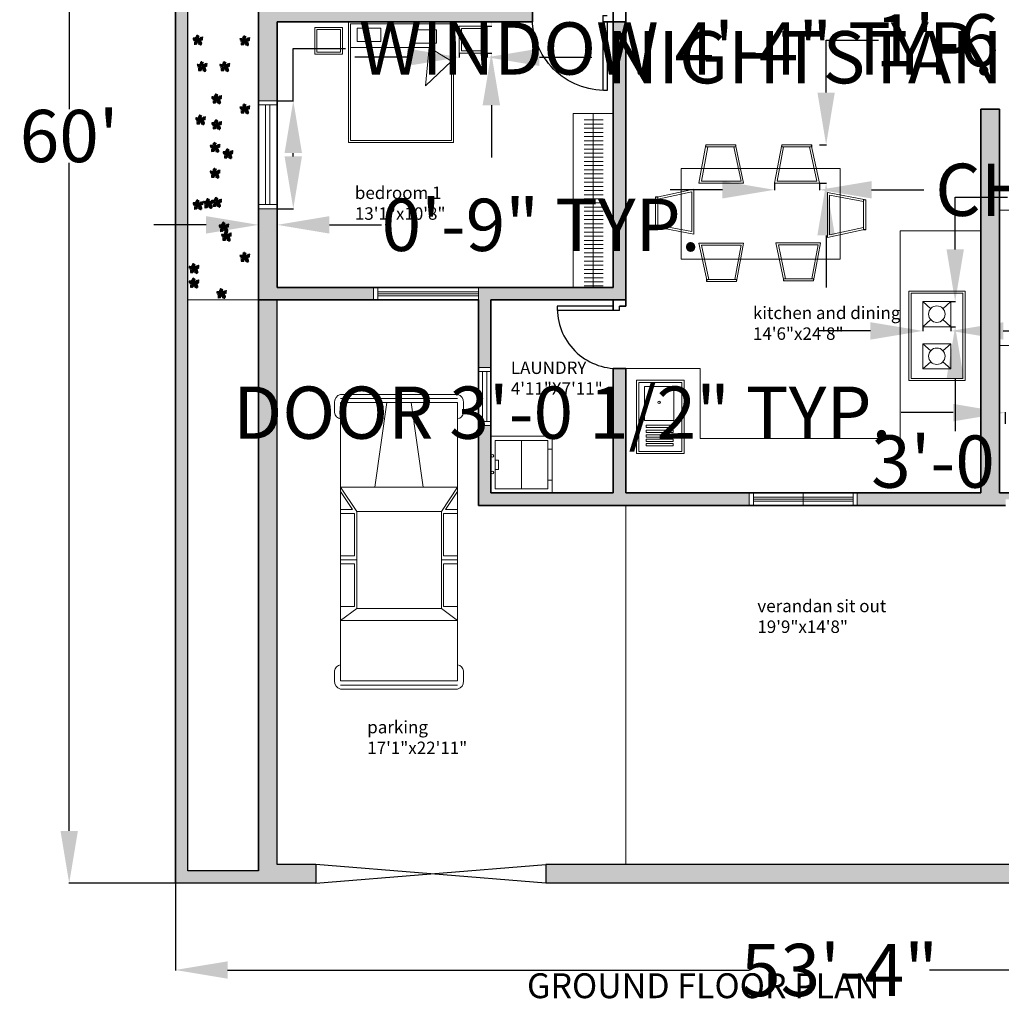
# Model space of a CAD drawing. Units: inches. Extents: x 23 to 3024, y 4 to 1405.
# Tile 1 of 7: x 2085 to 2558, y 518 to 992. Entities that reach past the tile are written whole.
import ezdxf

# ---------------------------------------------------------------- set-up
doc = ezdxf.new("R2010")
doc.units = ezdxf.units.IN
doc.header["$MEASUREMENT"] = 0
for name, color, linetype, lineweight in [('A-ANNO-DIMS', 2, 'Continuous', 18), ('A-ANNO-TEXT', 7, 'Continuous', 25), ('A-DOOR', 4, 'Continuous', 25), ('A-EQPM', 8, 'Continuous', 18), ('A-FLOR-CASE', 9, 'Continuous', 18), ('A-FLOR-FIXT', 9, 'Continuous', 18), ('A-WALL', 7, 'Continuous', 35), ('A-WALL-PATT', 189, 'Continuous', 13), ('C-PRKG-VEHC', 8, 'Continuous', 13), ('C-PROP', 7, 'Continuous', 30), ('C-SITE-GATE', 4, 'Continuous', 25), ('L-HRDS', 8, 'Continuous', 18), ('L-PLNT', 114, 'Continuous', 13)]:
    doc.layers.add(name, color=color, linetype=linetype, lineweight=lineweight)
for name, color, linetype, lineweight, true_color in [('A-AREA-IDEN', 30, 'Continuous', 18, 0xf8991e), ('A-FURN', 141, 'Continuous', 18, 0xadddf7), ('A-GLAZ', 30, 'Continuous', 18, 0xf26722)]:
    doc.layers.add(name, color=color, linetype=linetype, lineweight=lineweight, true_color=true_color)
doc.styles.get("Standard").update_dxf_attribs({"font": 'arial.ttf'})
doc.dimstyles.get("Standard").update_dxf_attribs({"dimtxt": 25.18, "dimasz": 25.18, "dimexe": 0.18, "dimexo": 0.0625, "dimgap": 0.09, "dimtad": 0, "dimtih": 1, "dimtoh": 1, "dimdec": 0, "dimrnd": 10, "dimzin": 0, "dimdsep": 46, "dimlunit": 3, "dimtxsty": 'Standard', "dimcen": 0.09, "dimadec": 0, "dimazin": 0, "dimtfac": 1, "dimtdec": 0, "dimtofl": 0, "dimtmove": 0, "dimatfit": 3, "dimfxl": 1, "dimtolj": 1, "dimtzin": 0, "dimarcsym": 0})

# ---------------------------------------------------------------- blocks, each defined once
blk = doc.blocks.new('*U4')
for p, q in [((5.44, 42.31), (12.12, 42.31)), ((189.69, 42.31), (183.01, 42.31)), ((0.1, -0.41), (0.1, 38.35)), ((2.77, -0.41), (2.77, 38.31)), ((5.44, -0.41), (5.44, 38.24)), ((5.45, 38.31), (16.12, 38.31)), ((16.12, 38.31), (180.34, 38.31)), ((61.52, -0.41), (61.52, 38.31)), ((61.52, 38.31), (77.54, 27.62)), ((64.19, 38.31), (76.2, 30.29)), ((76.2, 30.29), (76.2, 38.31)), ((78.87, 38.31), (78.87, 28.96)), ((106.91, 28.96), (106.91, 38.31)), ((109.58, 27.62), (109.58, 38.31)), ((112.25, 38.31), (112.25, 28.96)), ((140.29, 28.96), (140.29, 38.31)), ((141.62, 27.62), (149.64, 38.31)), ((149.64, -0.41), (149.64, 38.31)), ((189.69, 38.31), (179.01, 38.31)), ((189.69, -0.41), (189.69, 38.24)), ((192.36, -0.41), (192.36, 38.31)), ((195.03, -0.41), (195.03, 38.35)), ((77.54, 27.62), (141.62, 27.62)), ((77.54, -0.41), (77.54, 27.62)), ((78.87, 28.96), (106.91, 28.96)), ((112.25, 28.96), (140.29, 28.96)), ((141.62, -0.41), (141.62, 27.62)), ((5.44, 7.6), (61.52, 15.61)), ((0.1, -0.42), (0.1, -39.18)), ((2.77, -0.41), (2.77, -39.13)), ((5.44, -0.42), (5.44, -39.07)), ((61.52, -0.41), (61.52, -39.13)), ((77.54, -0.41), (77.54, -28.45)), ((141.62, -0.41), (141.62, -28.45)), ((149.64, -0.41), (149.64, -39.13)), ((189.69, -0.42), (189.69, -39.07)), ((192.36, -0.41), (192.36, -39.13)), ((195.03, -0.42), (195.03, -39.18)), ((5.44, -8.42), (61.52, -16.43)), ((61.52, -39.13), (77.54, -28.45)), ((64.19, -39.13), (76.2, -31.12)), ((76.2, -31.12), (76.2, -39.13)), ((77.54, -28.45), (141.62, -28.45)), ((78.87, -39.13), (78.87, -29.79)), ((78.87, -29.79), (106.91, -29.79)), ((106.91, -29.79), (106.91, -39.13)), ((109.58, -28.45), (109.58, -39.13)), ((112.25, -29.79), (140.29, -29.79)), ((112.25, -39.13), (112.25, -29.79)), ((140.29, -29.79), (140.29, -39.13)), ((141.62, -28.45), (149.64, -39.13)), ((5.44, -43.14), (12.12, -43.14)), ((5.45, -39.13), (16.12, -39.13)), ((16.12, -39.13), (180.34, -39.13)), ((189.69, -39.13), (179.01, -39.13)), ((189.69, -43.14), (183.01, -43.14))]:
    blk.add_line(p, q)
for centre, radius, start, end in [((5.06, 37.26), 5.06, 85.64554, 168.0943), ((11.45, 37.64), 4.72, 8.13011, 81.86996), ((183.68, 37.64), 4.72, 98.13004, 171.8699), ((190.07, 37.26), 5.06, 11.90574, 94.35446), ((5.06, -38.09), 5.06, 191.9057, 274.3545), ((11.45, -38.46), 4.72, 278.13, 351.8699), ((183.68, -38.46), 4.72, 188.1301, 261.87), ((190.07, -38.09), 5.06, 265.6455, 348.0943)]:
    blk.add_arc(centre, radius, start, end)
blk = doc.blocks.new('*U8')
for p, q in [((-47.498, 19.737), (-55.83, 18.344)), ((-40.615, 13.7), (-55.105, 10.913)), ((-31.5, 4.5), (-52.5, 25.5)), ((-33.37, 6.269), (-52.207, 5.34)), ((-48.585, 21.131), (-49.309, 29.026)), ((-28.299, 3.483), (-47.86, -5.805)), ((-43.513, 28.561), (-42.427, 15.558)), ((-38.442, 26.239), (-34.819, 7.663)), ((-21.416, 3.018), (-38.079, -8.128)), ((-35.544, 28.097), (-24.314, 3.947)), ((0, 0), (-31.5, 4.5)), ((-14.533, 2.09), (-30.834, 25.31)), ((-15.982, 2.09), (-30.11, -9.521)), ((-3.665, 19.273), (-27.574, 35.527)), ((-5.114, 28.097), (-24.676, 40.636)), ((-24.314, 23.917), (-2.941, 13.7)), ((0, 0), (-22.5, -19.5)), ((-7.288, 39.707), (-21.778, 46.673)), ((-6.563, 1.161), (-21.416, -8.128)), ((-20.691, 13.7), (-1.129, 4.876)), ((-8.737, 47.138), (-17.069, 52.711)), ((-10.186, 53.64), (-13.084, 55.962)), ((0, 0), (-10.5, 57)), ((-9.099, 51.782), (-6.563, 55.962)), ((-7.65, 43.423), (-2.578, 49.46)), ((-5.839, 35.992), (4.667, 48.067)), ((-5.114, 27.632), (10.463, 46.673)), ((-2.941, 16.486), (8.652, 37.85)), ((-1.129, 6.734), (9.014, 26.704)), ((0, 0), (27, 9)), ((0, 0), (18, -22.5)), ((3.942, 1.625), (11.187, 24.381)), ((6.478, 1.625), (26.04, -8.592)), ((10.101, 3.483), (17.708, 26.239)), ((11.187, 3.483), (30.749, -5.805)), ((16.259, 5.805), (23.142, 31.348)), ((18.07, 5.805), (35.096, -3.483)), ((22.055, 7.198), (27.489, 32.277)), ((24.229, 7.663), (46.688, 1.625)), ((27, 9), (48, 36)), ((27.127, 9.056), (31.112, 35.992)), ((29.662, 12.307), (48.137, 6.269)), ((31.836, 30.883), (32.561, 16.486)), ((33.285, 16.486), (48.862, 10.913)), ((35.096, 32.741), (37.27, 22.524)), ((36.183, 19.737), (48.137, 17.88)), ((38.719, 34.134), (41.979, 28.561)), ((40.53, 25.775), (48.862, 24.846)), ((43.791, 29.954), (51.036, 30.883)), ((44.153, 36.456), (45.239, 32.741)), ((-17.431, -15.094), (-42.789, -18.809)), ((-28.299, -29.026), (-42.789, -31.348)), ((-24.314, -21.596), (-42.427, -22.06)), ((-30.834, -34.135), (-42.427, -35.528)), ((-34.457, -39.708), (-40.978, -42.494)), ((-26.849, -26.24), (-40.253, -25.775)), ((-22.5, -19.5), (-37.5, -45)), ((-32.646, -36.921), (-31.921, -44.352)), ((-15.257, -12.772), (-30.11, -12.772)), ((-29.023, -30.884), (-27.936, -43.887)), ((-25.038, -23.918), (-22.865, -45.281)), ((-20.691, -18.345), (-17.793, -44.352)), ((-6.563, -5.805), (-19.967, -9.985)), ((-17.069, -15.094), (-12.721, -40.172)), ((-13.446, -11.378), (-8.737, -32.741)), ((-9.461, -8.592), (-6.201, -23.453)), ((-4.752, -3.483), (-3.665, -14.629)), ((2.493, -3.019), (-1.491, -20.202)), ((1.769, -2.555), (24.229, -9.521)), ((5.029, -6.27), (2.131, -25.775)), ((9.014, -11.378), (3.58, -35.992)), ((14.085, -16.951), (6.478, -40.172)), ((7.565, -9.056), (32.198, -14.629)), ((18.07, -22.524), (8.289, -45.745)), ((12.274, -15.094), (36.907, -18.809)), ((20.244, -30.419), (15.897, -44.816)), ((16.259, -19.738), (36.183, -22.989)), ((18, -22.5), (27, -52.5)), ((18.433, -22.524), (40.53, -29.026)), ((19.157, -25.311), (38.719, -33.206)), ((22.78, -37.85), (19.519, -48.532)), ((21.331, -32.741), (39.081, -40.636)), ((22.78, -38.314), (34.372, -44.816)), ((24.591, -45.745), (23.142, -50.854)), ((24.591, -43.423), (30.749, -47.603)), ((26.764, -49.925), (28.213, -50.854))]:
    blk.add_line(p, q)
blk = doc.blocks.new('*D10')
at = {"layer": 'A-ANNO-DIMS', "color": 0, "lineweight": -2, "transparency": 16777216}
for p, q in [((2160.39, 1295.93), (2109.1, 1295.93)), ((2109.28, 1270.75), (2109.28, 948.87)), ((2109.28, 601.11), (2109.28, 922.98)), ((2160.39, 575.93), (2109.1, 575.93))]:
    blk.add_line(p, q, dxfattribs=at)
at = {"layer": 'A-ANNO-DIMS', "color": 0, "transparency": 16777216}
for points in [[(2105.08, 1270.75), (2113.48, 1270.75), (2109.28, 1295.93)], [(2105.08, 601.11), (2113.48, 601.11), (2109.28, 575.93)]]:
    blk.add_solid(points, dxfattribs=at)
at = {"layer": 'Defpoints', "color": 0, "transparency": 16777216}
for p in [(2160.45, 1295.93), (2109.28, 575.93), (2160.45, 575.93)]:
    blk.add_point(p, dxfattribs=at)
at = {"layer": 'A-ANNO-DIMS', "color": 0, "transparency": 16777216, "insert": (2109.28, 935.93), "char_height": 25.18, "attachment_point": 5}
blk.add_mtext("\\A1;60'", dxfattribs=at)
blk = doc.blocks.new('CHAIR-DINING')
for p, q in [((0, 0), (3.44, 18.44)), ((1.2, 1), (4.27, 17.44)), ((3.44, 18.44), (17.66, 18.44)), ((4.27, 17.44), (16.85, 17.44)), ((16.85, 17.44), (20.33, 1)), ((17.66, 18.44), (21.56, 0)), ((20.33, 1), (1.2, 1)), ((21.56, 0), (0, 0))]:
    blk.add_line(p, q)
blk.add_lwpolyline([(3.44, 18.44), (17.88, 18.44), (17.88, 17.42), (3.44, 17.42)], close=True)
blk = doc.blocks.new('DOOR-SWING-36IN')
for p, q in [((-1, -1), (-1, 35)), ((1, 2), (1, 35)), ((-1, -1), (1, -1))]:
    blk.add_line(p, q)
blk.add_arc((0, 0), 35.01, 88.3634, 181.6366)
blk = doc.blocks.new('WINDOW-48IN')
for p, q in [((9, 52), (0, 52)), ((9, 50), (0, 50)), ((3.5, 2), (3.5, 50)), ((5.5, 2), (5.5, 50)), ((9, 2), (0, 2)), ((9, 0), (0, 0))]:
    blk.add_line(p, q)
blk = doc.blocks.new('COOKTOP-BURNER')
for p, q in [((0, 12.09), (3.84, 8.68)), ((13.6, 12.09), (9.76, 8.68)), ((0, 0), (3.84, 3.41)), ((13.6, 0), (9.76, 3.41))]:
    blk.add_line(p, q)
blk.add_lwpolyline([(0, 12.09), (13.6, 12.09), (13.6, 0), (0, 0)], close=True)
blk.add_circle((6.8, 6.05), 3.96)
blk = doc.blocks.new('NIGHTSTAND-SMALL')
for points in [[(0, 12.89), (13.42, 12.89), (13.42, 0), (0, 0)], [(1, 11.89), (12.42, 11.89), (12.42, 1), (1, 1)]]:
    blk.add_lwpolyline(points, close=True)
blk = doc.blocks.new('*D21')
at = {"layer": 'A-ANNO-DIMS', "color": 0, "lineweight": -2, "transparency": 16777216}
for p, q in [((2449.18, 913.2), (2449.18, 909.84)), ((2470.74, 913.2), (2470.74, 909.84)), ((2424, 910.02), (2398.82, 910.02)), ((2495.92, 910.02), (2521.1, 910.02))]:
    blk.add_line(p, q, dxfattribs=at)
at = {"layer": 'A-ANNO-DIMS', "color": 0, "transparency": 16777216}
for points in [[(2424, 914.22), (2424, 905.83), (2449.18, 910.02)], [(2495.92, 914.22), (2495.92, 905.83), (2470.74, 910.02)]]:
    blk.add_solid(points, dxfattribs=at)
at = {"layer": 'Defpoints', "color": 0, "transparency": 16777216}
for p in [(2449.18, 913.26), (2470.74, 913.26), (2470.74, 910.02)]:
    blk.add_point(p, dxfattribs=at)
at = {"layer": 'A-ANNO-DIMS', "color": 0, "transparency": 16777216, "insert": (2686.74, 910.02), "char_height": 25.18, "attachment_point": 5}
blk.add_mtext('\\A1;CHAIR 1\'-9 1/2" TYP.', dxfattribs=at)
blk = doc.blocks.new('*D22')
at = {"layer": 'A-ANNO-DIMS', "color": 0, "lineweight": -2, "transparency": 16777216}
for p, q in [((2473.98, 956.88), (2473.98, 982.06)), ((2473.98, 982.06), (2499.16, 982.06)), ((2470.81, 931.7), (2474.16, 931.7)), ((2470.81, 913.26), (2474.16, 913.26)), ((2473.98, 888.08), (2473.98, 862.9))]:
    blk.add_line(p, q, dxfattribs=at)
at = {"layer": 'A-ANNO-DIMS', "color": 0, "transparency": 16777216}
for points in [[(2469.78, 956.88), (2478.17, 956.88), (2473.98, 931.7)], [(2469.78, 888.08), (2478.17, 888.08), (2473.98, 913.26)]]:
    blk.add_solid(points, dxfattribs=at)
at = {"layer": 'Defpoints', "color": 0, "transparency": 16777216}
for p in [(2470.74, 931.7), (2473.98, 931.7), (2470.74, 913.26)]:
    blk.add_point(p, dxfattribs=at)
at = {"layer": 'A-ANNO-DIMS', "color": 0, "transparency": 16777216, "insert": (2604.14, 982.06), "char_height": 25.18, "attachment_point": 5}
blk.add_mtext('\\A1;1\'-6 1/2" TYP.', dxfattribs=at)
blk = doc.blocks.new('*D23')
at = {"layer": 'A-ANNO-DIMS', "color": 0, "lineweight": -2, "transparency": 16777216}
for p, q in [((2535.27, 802.64), (2510.09, 802.64)), ((2560.45, 797.26), (2560.45, 802.82)), ((2596.72, 797.26), (2596.72, 802.82)), ((2621.9, 802.64), (2647.08, 802.64))]:
    blk.add_line(p, q, dxfattribs=at)
at = {"layer": 'A-ANNO-DIMS', "color": 0, "transparency": 16777216}
for points in [[(2535.27, 806.84), (2535.27, 798.45), (2560.45, 802.64)], [(2621.9, 806.84), (2621.9, 798.45), (2596.72, 802.64)]]:
    blk.add_solid(points, dxfattribs=at)
at = {"layer": 'Defpoints', "color": 0, "transparency": 16777216}
for p in [(2560.45, 802.64), (2560.45, 797.2), (2596.72, 797.2)]:
    blk.add_point(p, dxfattribs=at)
at = {"layer": 'A-ANNO-DIMS', "color": 0, "transparency": 16777216, "insert": (2346.9, 802.64), "char_height": 25.18, "attachment_point": 5}
blk.add_mtext('\\A1;DOOR 3\'-0 1/2" TYP.', dxfattribs=at)
blk = doc.blocks.new('*D24')
at = {"layer": 'A-ANNO-DIMS', "color": 0, "lineweight": -2, "transparency": 16777216}
for p, q in [((2602.17, 822.38), (2602.17, 847.56)), ((2596.79, 797.2), (2602.35, 797.2)), ((2596.79, 760.93), (2602.35, 760.93)), ((2602.17, 735.75), (2602.17, 710.57))]:
    blk.add_line(p, q, dxfattribs=at)
at = {"layer": 'A-ANNO-DIMS', "color": 0, "transparency": 16777216}
for points in [[(2597.97, 822.38), (2606.36, 822.38), (2602.17, 797.2)], [(2597.97, 735.75), (2606.36, 735.75), (2602.17, 760.93)]]:
    blk.add_solid(points, dxfattribs=at)
at = {"layer": 'Defpoints', "color": 0, "transparency": 16777216}
for p in [(2596.72, 797.2), (2602.17, 797.2), (2596.72, 760.93)]:
    blk.add_point(p, dxfattribs=at)
at = {"layer": 'A-ANNO-DIMS', "color": 0, "transparency": 16777216, "insert": (2602.17, 779.06), "char_height": 25.18, "attachment_point": 5}
blk.add_mtext('\\A1;3\'-0 1/2" TYP.', dxfattribs=at)
blk = doc.blocks.new('*D27')
at = {"layer": 'A-ANNO-DIMS', "color": 0, "lineweight": -2, "transparency": 16777216}
for p, q in [((2217.25, 952.93), (2217.25, 978.11)), ((2217.25, 978.11), (2242.43, 978.11)), ((2209.51, 952.93), (2217.43, 952.93)), ((2217.25, 926.11), (2217.25, 927.75)), ((2209.51, 900.93), (2217.43, 900.93))]:
    blk.add_line(p, q, dxfattribs=at)
at = {"layer": 'A-ANNO-DIMS', "color": 0, "transparency": 16777216}
for points in [[(2213.05, 927.75), (2221.45, 927.75), (2217.25, 952.93)], [(2213.05, 926.11), (2221.45, 926.11), (2217.25, 900.93)]]:
    blk.add_solid(points, dxfattribs=at)
at = {"layer": 'Defpoints', "color": 0, "transparency": 16777216}
for p in [(2209.45, 952.93), (2217.25, 952.93), (2209.45, 900.93)]:
    blk.add_point(p, dxfattribs=at)
at = {"layer": 'A-ANNO-DIMS', "color": 0, "transparency": 16777216, "insert": (2401.83, 978.11), "char_height": 25.18, "attachment_point": 5}
blk.add_mtext('\\A1;WINDOW 4\'-4" TYP.', dxfattribs=at)
blk = doc.blocks.new('*D28')
at = {"layer": 'A-ANNO-DIMS', "color": 0, "lineweight": -2, "transparency": 16777216}
for p, q in [((2200.45, 900.86), (2200.45, 892.95)), ((2209.45, 900.86), (2209.45, 892.95)), ((2175.27, 893.13), (2150.09, 893.13)), ((2234.63, 893.13), (2259.81, 893.13))]:
    blk.add_line(p, q, dxfattribs=at)
at = {"layer": 'A-ANNO-DIMS', "color": 0, "transparency": 16777216}
for points in [[(2175.27, 897.32), (2175.27, 888.93), (2200.45, 893.13)], [(2234.63, 897.32), (2234.63, 888.93), (2209.45, 893.13)]]:
    blk.add_solid(points, dxfattribs=at)
at = {"layer": 'Defpoints', "color": 0, "transparency": 16777216}
for p in [(2200.45, 900.93), (2209.45, 900.93), (2209.45, 893.13)]:
    blk.add_point(p, dxfattribs=at)
at = {"layer": 'A-ANNO-DIMS', "color": 0, "transparency": 16777216, "insert": (2336.64, 893.13), "char_height": 25.18, "attachment_point": 5}
blk.add_mtext('\\A1;0\'-9" TYP.', dxfattribs=at)
blk = doc.blocks.new('*D33')
at = {"layer": 'A-ANNO-DIMS', "color": 0, "lineweight": -2, "transparency": 16777216}
for p, q in [((2495.35, 842.02), (2470.17, 842.02)), ((2520.53, 844), (2520.53, 841.84)), ((2534.13, 844), (2534.13, 841.84)), ((2559.31, 842.02), (2584.49, 842.02))]:
    blk.add_line(p, q, dxfattribs=at)
at = {"layer": 'A-ANNO-DIMS', "color": 0, "transparency": 16777216}
for points in [[(2495.35, 846.22), (2495.35, 837.83), (2520.53, 842.02)], [(2559.31, 846.22), (2559.31, 837.83), (2534.13, 842.02)]]:
    blk.add_solid(points, dxfattribs=at)
at = {"layer": 'Defpoints', "color": 0, "transparency": 16777216}
for p in [(2520.53, 844.06), (2534.13, 844.06), (2534.13, 842.02)]:
    blk.add_point(p, dxfattribs=at)
at = {"layer": 'A-ANNO-DIMS', "color": 0, "transparency": 16777216, "insert": (2769.25, 842.02), "char_height": 25.18, "attachment_point": 5}
blk.add_mtext('\\A1;BURNER 1\'-1 1/2" TYP.', dxfattribs=at)
blk = doc.blocks.new('*D34')
at = {"layer": 'A-ANNO-DIMS', "color": 0, "lineweight": -2, "transparency": 16777216}
for p, q in [((2536.16, 881.33), (2536.16, 906.51)), ((2536.16, 906.51), (2561.34, 906.51)), ((2534.19, 856.15), (2536.34, 856.15)), ((2534.19, 844.06), (2536.34, 844.06)), ((2536.16, 818.88), (2536.16, 793.7))]:
    blk.add_line(p, q, dxfattribs=at)
at = {"layer": 'A-ANNO-DIMS', "color": 0, "transparency": 16777216}
for points in [[(2531.97, 881.33), (2540.36, 881.33), (2536.16, 856.15)], [(2531.97, 818.88), (2540.36, 818.88), (2536.16, 844.06)]]:
    blk.add_solid(points, dxfattribs=at)
at = {"layer": 'Defpoints', "color": 0, "transparency": 16777216}
for p in [(2534.13, 856.15), (2536.16, 856.15), (2534.13, 844.06)]:
    blk.add_point(p, dxfattribs=at)
at = {"layer": 'A-ANNO-DIMS', "color": 0, "transparency": 16777216, "insert": (2636.99, 906.51), "char_height": 25.18, "attachment_point": 5}
blk.add_mtext('\\A1;1\'-0" TYP.', dxfattribs=at)
blk = doc.blocks.new('*D35')
at = {"layer": 'A-ANNO-DIMS', "color": 0, "lineweight": -2, "transparency": 16777216}
for p, q in [((2272.06, 973.9), (2246.88, 973.9)), ((2297.24, 975.85), (2297.24, 973.72)), ((2310.67, 975.85), (2310.67, 973.72)), ((2335.85, 973.9), (2361.03, 973.9))]:
    blk.add_line(p, q, dxfattribs=at)
at = {"layer": 'A-ANNO-DIMS', "color": 0, "transparency": 16777216}
for points in [[(2272.06, 978.09), (2272.06, 969.7), (2297.24, 973.9)], [(2335.85, 978.09), (2335.85, 969.7), (2310.67, 973.9)]]:
    blk.add_solid(points, dxfattribs=at)
at = {"layer": 'Defpoints', "color": 0, "transparency": 16777216}
for p in [(2297.24, 975.91), (2310.67, 975.91), (2310.67, 973.9)]:
    blk.add_point(p, dxfattribs=at)
at = {"layer": 'A-ANNO-DIMS', "color": 0, "transparency": 16777216, "insert": (2585.8, 973.9), "char_height": 25.18, "attachment_point": 5}
blk.add_mtext('\\A1;NIGHTSTAND 1\'-1 1/2" TYP.', dxfattribs=at)
blk = doc.blocks.new('*D36')
at = {"layer": 'A-ANNO-DIMS', "color": 0, "lineweight": -2, "transparency": 16777216}
for p, q in [((2312.68, 1013.98), (2312.68, 1039.16)), ((2312.68, 1039.16), (2337.86, 1039.16)), ((2310.73, 988.8), (2312.86, 988.8)), ((2310.73, 975.91), (2312.86, 975.91)), ((2312.68, 950.73), (2312.68, 925.55))]:
    blk.add_line(p, q, dxfattribs=at)
at = {"layer": 'A-ANNO-DIMS', "color": 0, "transparency": 16777216}
for points in [[(2308.48, 1013.98), (2316.88, 1013.98), (2312.68, 988.8)], [(2308.48, 950.73), (2316.88, 950.73), (2312.68, 975.91)]]:
    blk.add_solid(points, dxfattribs=at)
at = {"layer": 'Defpoints', "color": 0, "transparency": 16777216}
for p in [(2310.67, 988.8), (2312.68, 988.8), (2310.67, 975.91)]:
    blk.add_point(p, dxfattribs=at)
at = {"layer": 'A-ANNO-DIMS', "color": 0, "transparency": 16777216, "insert": (2413.51, 1039.16), "char_height": 25.18, "attachment_point": 5}
blk.add_mtext('\\A1;1\'-1" TYP.', dxfattribs=at)
blk = doc.blocks.new('*D37')
at = {"layer": 'A-ANNO-DIMS', "color": 0, "lineweight": -2, "transparency": 16777216}
for p, q in [((2214.42, 1078.46), (2214.42, 1076)), ((2230.01, 1078.46), (2230.01, 1076)), ((2189.24, 1076.18), (2164.06, 1076.18)), ((2255.19, 1076.18), (2280.37, 1076.18))]:
    blk.add_line(p, q, dxfattribs=at)
at = {"layer": 'A-ANNO-DIMS', "color": 0, "transparency": 16777216}
for points in [[(2189.24, 1080.38), (2189.24, 1071.99), (2214.42, 1076.18)], [(2255.19, 1080.38), (2255.19, 1071.99), (2230.01, 1076.18)]]:
    blk.add_solid(points, dxfattribs=at)
at = {"layer": 'Defpoints', "color": 0, "transparency": 16777216}
for p in [(2214.42, 1078.52), (2230.01, 1078.52), (2230.01, 1076.18)]:
    blk.add_point(p, dxfattribs=at)
at = {"layer": 'A-ANNO-DIMS', "color": 0, "transparency": 16777216, "insert": (2499.37, 1076.18), "char_height": 25.18, "attachment_point": 5}
blk.add_mtext('\\A1;LAMP TABLE 1\'-3 1/2" TYP.', dxfattribs=at)
blk = doc.blocks.new('*D41')
at = {"layer": 'A-ANNO-DIMS', "color": 0, "lineweight": -2, "transparency": 16777216}
for p, q in [((2160.45, 575.86), (2160.45, 533.9)), ((2800.45, 575.86), (2800.45, 533.9)), ((2185.63, 534.08), (2437.11, 534.08)), ((2775.27, 534.08), (2523.79, 534.08))]:
    blk.add_line(p, q, dxfattribs=at)
at = {"layer": 'A-ANNO-DIMS', "color": 0, "transparency": 16777216}
for points in [[(2185.63, 538.27), (2185.63, 529.88), (2160.45, 534.08)], [(2775.27, 538.27), (2775.27, 529.88), (2800.45, 534.08)]]:
    blk.add_solid(points, dxfattribs=at)
at = {"layer": 'Defpoints', "color": 0, "transparency": 16777216}
for p in [(2160.45, 575.93), (2800.45, 575.93), (2800.45, 534.08)]:
    blk.add_point(p, dxfattribs=at)
at = {"layer": 'A-ANNO-DIMS', "color": 0, "transparency": 16777216, "insert": (2480.45, 534.08), "char_height": 25.18, "attachment_point": 5}
blk.add_mtext('\\A1;53\'-4"', dxfattribs=at)

msp = doc.modelspace()

# ---------------------------------------------------------------- hatches: boundary and pattern name
at = {"layer": 'A-WALL-PATT'}
h = msp.add_hatch(color=256, dxfattribs=at)
h.dxf.hatch_style = 1
h.paths.add_polyline_path([(2209.45, 1233.93), (2200.45, 1233.93), (2200.45, 1160.43), (2209.45, 1160.43), (2209.45, 1167.77), (2209.45, 1202.93), (2306.45, 1202.93), (2306.45, 1208.93), (2300.45, 1208.93), (2209.45, 1208.93)], flags=17)
h.paths.add_polyline_path([(2800.45, 1295.93), (2200.45, 1295.93), (2160.45, 1295.93), (2160.45, 575.93), (2200.45, 575.93), (2228.06, 575.93), (2228.06, 584.93), (2209.45, 584.93), (2209.45, 856.93), (2200.45, 856.93), (2200.45, 581.93), (2166.45, 581.93), (2166.45, 1289.93), (2200.45, 1289.93), (2200.45, 1261.93), (2209.45, 1261.93), (2209.45, 1286.93), (2244.45, 1286.93), (2300.45, 1286.93), (2300.45, 1241.93), (2301.45, 1241.93, -0.017236), (2303.45, 1241.93), (2306.45, 1241.93), (2306.45, 1286.93), (2548.45, 1286.93), (2548.45, 1261.93), (2557.45, 1261.93), (2557.45, 1286.93), (2791.45, 1286.93), (2791.45, 1140.93), (2613.74, 1140.93), (2613.74, 1134.93), (2791.45, 1134.93), (2791.45, 927.1), (2800.45, 927.1)])
h.paths.add_polyline_path([(2166.06, 1284.53), (2166.03, 1284.87), (2166.29, 1284.91), (2166.32, 1284.58)], flags=16)
h.paths.add_polyline_path([(2557.45, 1233.93), (2548.45, 1233.93), (2548.45, 1208.93), (2514.78, 1208.93), (2457.45, 1208.93), (2451.45, 1208.93), (2451.45, 1202.93), (2548.45, 1202.93), (2557.45, 1202.93)], flags=17)
h.paths.add_polyline_path([(2457.45, 1286.93), (2451.45, 1286.93), (2451.45, 1241.93), (2454.45, 1241.93, -0.017236), (2456.45, 1241.93), (2457.45, 1241.93)], flags=17)
h.paths.add_polyline_path([(2419.96, 1208.93), (2378.45, 1208.93), (2378.45, 1286.93), (2372.45, 1286.93), (2372.45, 1208.93), (2352.45, 1208.93), (2352.45, 1202.93), (2419.96, 1202.93)], flags=17)
h.paths.add_polyline_path([(2557.45, 1134.93), (2563.84, 1134.93), (2563.84, 1140.93), (2557.45, 1140.93), (2557.45, 1149.12), (2548.45, 1149.12), (2548.45, 1103.07), (2548.45, 1065.93), (2416.45, 1065.93), (2416.45, 1064.93, -0.014283), (2416.45, 1062.93), (2416.45, 1059.93), (2548.45, 1059.93), (2548.45, 1025.12), (2557.45, 1025.12)], flags=17)
h.paths.add_polyline_path([(2332.45, 1062.93, -0.014283), (2332.45, 1064.93), (2332.45, 1065.93), (2209.45, 1065.93), (2209.45, 1108.43), (2200.45, 1108.43), (2200.45, 1042.43), (2209.45, 1042.43), (2209.45, 1059.93), (2332.45, 1059.93)], flags=17)
h.paths.add_polyline_path([(2332.45, 996.93), (2209.45, 996.93), (2209.45, 1014.43), (2200.45, 1014.43), (2200.45, 952.93), (2209.45, 952.93), (2209.45, 990.93), (2332.45, 990.93), (2332.45, 991.93, -0.014283), (2332.45, 993.93)], flags=17)
h.paths.add_polyline_path([(2209.45, 900.93), (2200.45, 900.93), (2200.45, 856.93), (2209.45, 856.93), (2255.95, 856.93), (2255.95, 862.93), (2209.45, 862.93)], flags=17)
h.paths.add_polyline_path([(2377.45, 823.93), (2374.45, 823.93, -0.017236), (2372.45, 823.93), (2371.45, 823.93), (2371.45, 763.93), (2312.45, 763.93), (2312.45, 791.27), (2312.45, 796.43), (2306.45, 796.43), (2306.45, 757.93), (2436.95, 757.93), (2436.95, 763.93), (2377.45, 763.93)], flags=17)
h.paths.add_polyline_path([(2557.45, 948.81), (2548.45, 948.81), (2548.45, 763.93), (2488.95, 763.93), (2488.95, 757.93), (2560.45, 757.93), (2560.45, 760.93), (2562.45, 760.93), (2562.45, 763.93), (2557.45, 763.93)], flags=17)
h.paths.add_polyline_path([(2377.45, 990.93), (2371.45, 990.93), (2371.45, 862.93), (2306.45, 862.93), (2306.45, 856.93), (2306.45, 824.43), (2312.45, 824.43), (2312.45, 856.93), (2371.45, 856.93), (2377.45, 856.93)], flags=17)
h.paths.add_polyline_path([(2800.45, 875.1), (2791.45, 875.1), (2791.45, 763.93), (2719.93, 763.93), (2719.93, 757.93), (2791.45, 757.93), (2791.45, 584.93), (2338.88, 584.93), (2338.88, 575.93), (2800.45, 575.93)], flags=17)
h.paths.add_polyline_path([(2667.93, 763.93), (2596.45, 763.93), (2596.45, 762.93, -0.014283), (2596.45, 760.93), (2596.45, 757.93), (2667.93, 757.93)], flags=16)

# ---------------------------------------------------------------- linework, layer by layer
at = {"layer": 'A-DOOR'}
msp.add_line((2374.45, 851.93), (2374.45, 853.93), dxfattribs=at)
for points in [[(2371.45, 853.93), (2344.45, 853.93)], [(2374.45, 851.93), (2344.45, 851.93)]]:
    msp.add_lwpolyline(points, dxfattribs=at)
msp.add_arc((2373.45, 852.93), 29.02, 178.0251, 271.9749, dxfattribs=at)
at = {"layer": 'A-EQPM'}
for p, q in [((2327.2, 789.27), (2327.2, 765.93)), ((2341.95, 785.12), (2339.95, 785.12)), ((2314.45, 779.81), (2316.06, 779.81)), ((2316.06, 779.81), (2316.06, 775.2)), ((2316.06, 775.2), (2314.45, 775.2)), ((2341.95, 770.06), (2339.95, 770.06))]:
    msp.add_line(p, q, dxfattribs=at)
for points in [[(2557.45, 900.13), (2574.69, 900.13), (2574.69, 834.99), (2557.45, 834.99)], [(2540.9, 861.25), (2513.89, 861.25), (2513.89, 818.14), (2540.9, 818.14)], [(2539.9, 860.25), (2514.89, 860.25), (2514.89, 819.14), (2539.9, 819.14)], [(2312.45, 791.27), (2341.95, 791.27), (2341.95, 763.93), (2312.45, 763.93)], [(2314.45, 789.27), (2339.95, 789.27), (2339.95, 765.93), (2314.45, 765.93)]]:
    msp.add_lwpolyline(points, close=True, dxfattribs=at)
for centre in [(2313.18, 781.8), (2313.18, 773.84)]:
    msp.add_circle(centre, 0.641, dxfattribs=at)
at = {"layer": 'A-FLOR-CASE'}
for p, q in [((2371.45, 946.73), (2352.18, 946.73)), ((2352.18, 946.73), (2352.18, 862.93)), ((2361.82, 946.73), (2361.82, 862.93)), ((2509.65, 790.25), (2509.65, 890.29)), ((2509.65, 890.29), (2548.45, 890.29)), ((2377.45, 823.93), (2413.37, 823.93)), ((2413.37, 823.93), (2413.37, 790.25)), ((2413.37, 790.25), (2509.65, 790.25))]:
    msp.add_line(p, q, dxfattribs=at)
for points in [[(2357.42, 943.67), (2366.51, 943.67)], [(2357.42, 941.67), (2366.51, 941.67)], [(2357.42, 939.67), (2366.51, 939.67)], [(2357.42, 937.67), (2366.51, 937.67)], [(2357.42, 935.67), (2366.51, 935.67)], [(2357.42, 933.67), (2366.51, 933.67)], [(2357.42, 931.67), (2366.51, 931.67)], [(2357.42, 929.67), (2366.51, 929.67)], [(2357.42, 927.67), (2366.51, 927.67)], [(2357.42, 925.67), (2366.51, 925.67)], [(2357.42, 923.67), (2366.51, 923.67)], [(2357.42, 921.67), (2366.51, 921.67)], [(2357.42, 919.67), (2366.51, 919.67)], [(2357.42, 917.67), (2366.51, 917.67)], [(2357.42, 915.67), (2366.51, 915.67)], [(2357.42, 913.67), (2366.51, 913.67)], [(2357.42, 911.67), (2366.51, 911.67)], [(2357.42, 909.67), (2366.51, 909.67)], [(2357.42, 907.67), (2366.51, 907.67)], [(2357.42, 905.67), (2366.51, 905.67)], [(2357.42, 903.67), (2366.51, 903.67)], [(2357.42, 901.67), (2366.51, 901.67)], [(2357.42, 899.67), (2366.51, 899.67)], [(2357.42, 897.67), (2366.51, 897.67)], [(2357.42, 895.67), (2366.51, 895.67)], [(2357.42, 893.67), (2366.51, 893.67)], [(2357.42, 891.67), (2366.51, 891.67)], [(2357.42, 889.67), (2366.51, 889.67)], [(2357.42, 887.67), (2366.51, 887.67)], [(2357.42, 885.67), (2366.51, 885.67)], [(2357.42, 883.67), (2366.51, 883.67)], [(2357.42, 881.67), (2366.51, 881.67)], [(2357.42, 879.67), (2366.51, 879.67)], [(2357.42, 877.67), (2366.51, 877.67)], [(2357.42, 875.67), (2366.51, 875.67)], [(2357.42, 873.67), (2366.51, 873.67)], [(2357.42, 871.67), (2366.51, 871.67)], [(2357.42, 869.67), (2366.51, 869.67)], [(2357.42, 867.67), (2366.51, 867.67)], [(2357.42, 865.67), (2366.51, 865.67)], [(2357.42, 863.67), (2366.51, 863.67)]]:
    msp.add_lwpolyline(points, dxfattribs=at)
at = {"layer": 'A-FLOR-FIXT'}
for points in [[(2382.69, 818.25), (2405.53, 818.25), (2405.53, 782.93), (2382.69, 782.93)], [(2383.69, 817.25), (2404.53, 817.25), (2404.53, 783.93), (2383.69, 783.93)], [(2386.44, 815.24), (2400.67, 815.24), (2400.67, 798.8), (2386.44, 798.8)], [(2387.23, 796.55), (2400.33, 796.55), (2400.33, 795.48), (2387.23, 795.48)], [(2387.23, 794.21), (2400.33, 794.21), (2400.33, 793.13), (2387.23, 793.13)], [(2387.23, 791.96), (2400.33, 791.96), (2400.33, 790.89), (2387.23, 790.89)], [(2387.23, 789.82), (2400.33, 789.82), (2400.33, 788.74), (2387.23, 788.74)], [(2387.23, 787.77), (2400.33, 787.77), (2400.33, 786.69), (2387.23, 786.69)]]:
    msp.add_lwpolyline(points, close=True, dxfattribs=at)
msp.add_circle((2393.51, 807.6), 0.6, dxfattribs=at)
at = {"layer": 'A-FURN'}
for p, q in [((2244.81, 978.62), (2282.75, 978.62)), ((2281, 960.04), (2282.75, 978.62)), ((2282.75, 978.62), (2293.45, 972.06)), ((2293.45, 972.06), (2281, 960.04)), ((2413.96, 920.24), (2432.74, 920.24))]:
    msp.add_line(p, q, dxfattribs=at)
for points in [[(2243.81, 990.93), (2294.45, 990.93), (2294.45, 932.81), (2243.81, 932.81)], [(2244.81, 989.93), (2293.45, 989.93), (2293.45, 933.81), (2244.81, 933.81)], [(2248.01, 987.87), (2259.44, 987.87), (2259.44, 981.42), (2248.01, 981.42)], [(2274.89, 987.06), (2286.32, 987.06), (2286.32, 980.61), (2274.89, 980.61)]]:
    msp.add_lwpolyline(points, close=True, dxfattribs=at)
msp.add_lwpolyline([(2432.74, 920.24), (2480.72, 920.24), (2480.72, 876.58), (2404.06, 876.58), (2404.06, 920.24), (2413.96, 920.24)], dxfattribs=at)
at = {"layer": 'A-GLAZ'}
for p, q in [((2255.95, 856.93), (2255.95, 862.93)), ((2257.95, 856.93), (2257.95, 862.93)), ((2306.45, 860.93), (2257.95, 860.93)), ((2306.45, 859.93), (2257.95, 859.93)), ((2306.45, 858.93), (2257.95, 858.93)), ((2306.45, 856.93), (2306.45, 862.93)), ((2312.45, 824.43), (2306.45, 824.43)), ((2312.45, 822.43), (2306.45, 822.43)), ((2308.45, 822.43), (2308.45, 798.43)), ((2310.45, 822.43), (2310.45, 798.43)), ((2310.45, 822.43), (2310.45, 798.43)), ((2312.45, 798.43), (2306.45, 798.43)), ((2312.45, 796.43), (2306.45, 796.43)), ((2436.95, 763.93), (2436.95, 757.93)), ((2438.95, 763.93), (2438.95, 757.93)), ((2462.95, 763.93), (2462.95, 757.93)), ((2486.95, 763.93), (2486.95, 757.93)), ((2488.95, 763.93), (2488.95, 757.93)), ((2438.95, 761.93), (2486.95, 761.93)), ((2438.95, 760.93), (2486.95, 760.93)), ((2438.95, 759.93), (2486.95, 759.93))]:
    msp.add_line(p, q, dxfattribs=at)
at = {"layer": 'A-WALL'}
for p, q in [((2200.45, 581.93), (2200.45, 1289.93)), ((2332.45, 996.93), (2332.45, 990.93)), ((2371.45, 996.93), (2371.45, 862.93)), ((2377.45, 996.93), (2377.45, 856.93)), ((2209.45, 990.93), (2332.49, 990.93)), ((2209.45, 862.93), (2209.45, 990.93)), ((2366.45, 990.93), (2377.45, 990.93)), ((2548.45, 948.81), (2557.45, 948.81)), ((2548.45, 948.81), (2548.45, 763.93)), ((2557.45, 948.81), (2557.45, 763.93)), ((2209.45, 862.93), (2371.45, 862.93)), ((2209.45, 856.93), (2200.45, 856.93)), ((2209.45, 856.93), (2306.45, 856.93)), ((2306.45, 856.93), (2306.45, 757.93)), ((2312.45, 856.93), (2312.45, 763.93)), ((2312.45, 856.93), (2371.45, 856.93)), ((2371.45, 856.93), (2371.45, 851.93)), ((2371.45, 856.93), (2377.45, 856.93)), ((2377.45, 856.93), (2377.45, 853.93)), ((2374.45, 853.93), (2377.45, 853.93)), ((2371.45, 823.98), (2371.45, 763.93)), ((2371.45, 823.93), (2377.45, 823.93)), ((2377.45, 823.93), (2377.45, 763.93)), ((2312.45, 763.93), (2371.45, 763.93)), ((2377.45, 763.93), (2548.45, 763.93)), ((2557.45, 763.93), (2562.45, 763.93)), ((2306.45, 757.93), (2560.45, 757.93))]:
    msp.add_line(p, q, dxfattribs=at)
at = {"layer": 'C-PROP'}
for p, q in [((2160.45, 575.93), (2160.45, 1295.93)), ((2160.45, 1295.93), (2160.45, 575.93)), ((2166.45, 581.93), (2166.45, 1289.93)), ((2209.45, 584.93), (2209.45, 856.93)), ((2228.06, 584.93), (2209.45, 584.93)), ((2791.45, 584.93), (2338.88, 584.93)), ((2200.45, 581.93), (2166.45, 581.93)), ((2200.45, 575.93), (2160.45, 575.93)), ((2228.06, 575.93), (2200.45, 575.93)), ((2800.45, 575.93), (2338.88, 575.93))]:
    msp.add_line(p, q, dxfattribs=at)
at = {"layer": 'C-SITE-GATE'}
for p, q in [((2228.06, 584.93), (2228.06, 575.93)), ((2338.88, 575.93), (2228.06, 584.93)), ((2228.06, 575.93), (2338.88, 584.93)), ((2338.88, 584.93), (2338.88, 575.93)), ((2228.06, 575.93), (2228.06, 575.93))]:
    msp.add_line(p, q, dxfattribs=at)
at = {"layer": 'L-HRDS'}
for p, q in [((2200.45, 856.93), (2166.45, 856.93)), ((2377.45, 757.93), (2377.45, 584.93))]:
    msp.add_line(p, q, dxfattribs=at)

# ---------------------------------------------------------------- block references
at = {"layer": 'A-DOOR', "extrusion": (0, 0, -1), "zscale": -1, "rotation": 180}
msp.add_blockref('DOOR-SWING-36IN', (-2367.45, 992.93), dxfattribs=at)
at = {"layer": 'A-EQPM'}
for p in [(2520.53, 844.06), (2520.53, 823.78)]:
    msp.add_blockref('COOKTOP-BURNER', p, dxfattribs=at)
at = {"layer": 'A-FURN'}
for name, p in [('NIGHTSTAND-SMALL', (2227.6, 975.33)), ('NIGHTSTAND-SMALL', (2297.24, 975.91)), ('CHAIR-DINING', (2412.66, 913.26)), ('CHAIR-DINING', (2449.18, 913.26))]:
    msp.add_blockref(name, p, dxfattribs=at)
for p, rotation in [((2410.29, 888.69), 89.99999999999365), ((2474.61, 908.67), 269.9999999999959), ((2434.25, 884.3), 180), ((2471.31, 884.52), 180)]:
    msp.add_blockref('CHAIR-DINING', p, dxfattribs=dict(at, rotation=rotation))
at = {"layer": 'A-GLAZ'}
msp.add_blockref('WINDOW-48IN', (2200.45, 900.93), dxfattribs=at)
at = {"layer": 'C-PRKG-VEHC', "xscale": 0.7281375025229884, "yscale": 0.7281375025229884, "zscale": 0.7281375025229884, "rotation": 270}
msp.add_blockref('*U4', (2268.52, 811.46), dxfattribs=at)
at = {"layer": 'L-PLNT', "xscale": 0.0466330202614855, "yscale": 0.0466330202614855, "zscale": 0.0466330202614855}
for p in [(2171.42, 982.05), (2194.03, 981.76), (2173.47, 969.3), (2184.39, 969.3), (2180.49, 953.73), (2194.03, 948.88), (2172.69, 943.6), (2180.49, 941.27), (2179.71, 930.36), (2185.95, 927.25), (2179.71, 917.9), (2180.49, 903.89), (2171.47, 902.7), (2176.45, 903.28), (2183.99, 891.92), (2185.17, 887.53), (2194.03, 877.41), (2169.57, 871.96), (2169.57, 864.95), (2182.84, 859.9)]:
    msp.add_blockref('*U8', p, dxfattribs=at)

# ---------------------------------------------------------------- texts
at = {"layer": 'A-ANNO-TEXT', "insert": (2329.87, 532.5), "char_height": 12, "attachment_point": 1}
msp.add_mtext_dynamic_manual_height_columns('GROUND FLOOR PLAN', width=495.577, gutter_width=1, heights=[0], dxfattribs=at)
at = {"layer": 'A-AREA-IDEN', "char_height": 6, "attachment_point": 1}
for s, width, insert in [('bedroom 1\\P13\'1"x10\'8"', 46.8839, (2246.94, 911.58)), ('kitchen and dining\\P14\'6"x24\'8"', 71.1641, (2438.72, 853.73)), ('LAUNDRY\\P4\'11"X7\'11"', 46.8839, (2322.08, 827.28)), ('verandan sit out\\P19\'9"x14\'8"', 71.1641, (2440.85, 712.5)), ('parking \\P17\'1"x22\'11"', 71.1641, (2252.89, 654.12))]:
    msp.add_mtext_dynamic_manual_height_columns(s, width=width, gutter_width=1, heights=[0], dxfattribs=dict(at, insert=insert))

# ---------------------------------------------------------------- dimensions: what is measured, and where the dimension line sits
at = {"layer": 'A-ANNO-DIMS'}
dim = msp.add_linear_dim(base=(2109.28, 575.93), p1=(2160.45, 1295.93), p2=(2160.45, 575.93), angle=90, dimstyle='Standard', override={"dimclrd": 0, "dimclre": 0, "dimclrt": 0}, dxfattribs=at)
dim.commit()
dim.dimension.update_dxf_attribs({"geometry": '*D10', "text_midpoint": (2109.28, 935.93)})
for base, p1, p2, text, picture, middle in [((2230.01, 1076.18), (2214.42, 1078.52), (2230.01, 1078.52), 'LAMP TABLE <> TYP.', '*D37', (2499.37, 1076.18)), ((2310.67, 973.9), (2297.24, 975.91), (2310.67, 975.91), 'NIGHTSTAND <> TYP.', '*D35', (2585.8, 973.9)), ((2470.74, 910.02), (2449.18, 913.26), (2470.74, 913.26), 'CHAIR <> TYP.', '*D21', (2686.74, 910.02)), ((2209.45, 893.13), (2200.45, 900.93), (2209.45, 900.93), '<> TYP.', '*D28', (2336.64, 893.13)), ((2534.13, 842.02), (2520.53, 844.06), (2534.13, 844.06), 'BURNER <> TYP.', '*D33', (2769.25, 842.02))]:
    dim = msp.add_linear_dim(base=base, p1=p1, p2=p2, text=text, dimstyle='Standard', override={"dimdec": 1, "dimlfac": 1, "dimrnd": 0, "dimzin": 1, "dimdsep": 46, "dimlunit": 4, "dimfrac": 2}, dxfattribs=at)
    dim.commit()
    dim.dimension.update_dxf_attribs({"geometry": picture, "text_midpoint": middle})
for base, p1, p2, angle, text, picture, middle in [((2312.68, 988.8), (2310.67, 975.91), (2310.67, 988.8), 90, '<> TYP.', '*D36', (2413.51, 1039.16)), ((2473.98, 931.7), (2470.74, 913.26), (2470.74, 931.7), 90, '<> TYP.', '*D22', (2604.14, 982.06)), ((2217.25, 952.93), (2209.45, 900.93), (2209.45, 952.93), 90, 'WINDOW <> TYP.', '*D27', (2401.83, 978.11)), ((2536.16, 856.15), (2534.13, 844.06), (2534.13, 856.15), 90, '<> TYP.', '*D34', (2636.99, 906.51)), ((2560.45, 802.64), (2596.72, 797.2), (2560.45, 797.2), 180, 'DOOR <> TYP.', '*D23', (2346.9, 802.64)), ((2602.17, 797.2), (2596.72, 760.93), (2596.72, 797.2), 90, '<> TYP.', '*D24', (2602.17, 779.06))]:
    dim = msp.add_linear_dim(base=base, p1=p1, p2=p2, angle=angle, text=text, dimstyle='Standard', override={"dimdec": 1, "dimlfac": 1, "dimrnd": 0, "dimzin": 1, "dimdsep": 46, "dimlunit": 4, "dimfrac": 2}, dxfattribs=at)
    dim.commit()
    dim.dimension.update_dxf_attribs({"geometry": picture, "text_midpoint": middle})
dim = msp.add_linear_dim(base=(2800.45, 534.08), p1=(2160.45, 575.93), p2=(2800.45, 575.93), dimstyle='Standard', override={"dimdec": 1, "dimlfac": 1, "dimrnd": 0, "dimzin": 1, "dimdsep": 46, "dimlunit": 4, "dimfrac": 2}, dxfattribs=at)
dim.commit()
dim.dimension.update_dxf_attribs({"geometry": '*D41', "text_midpoint": (2480.45, 534.08)})

doc.saveas('drawing.dxf')
